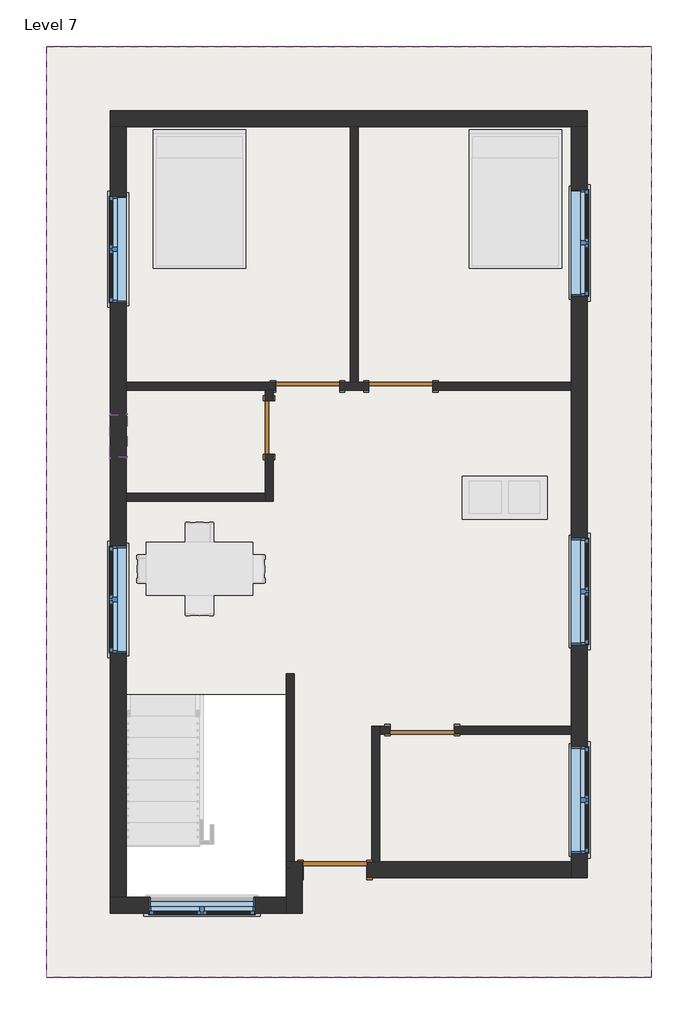
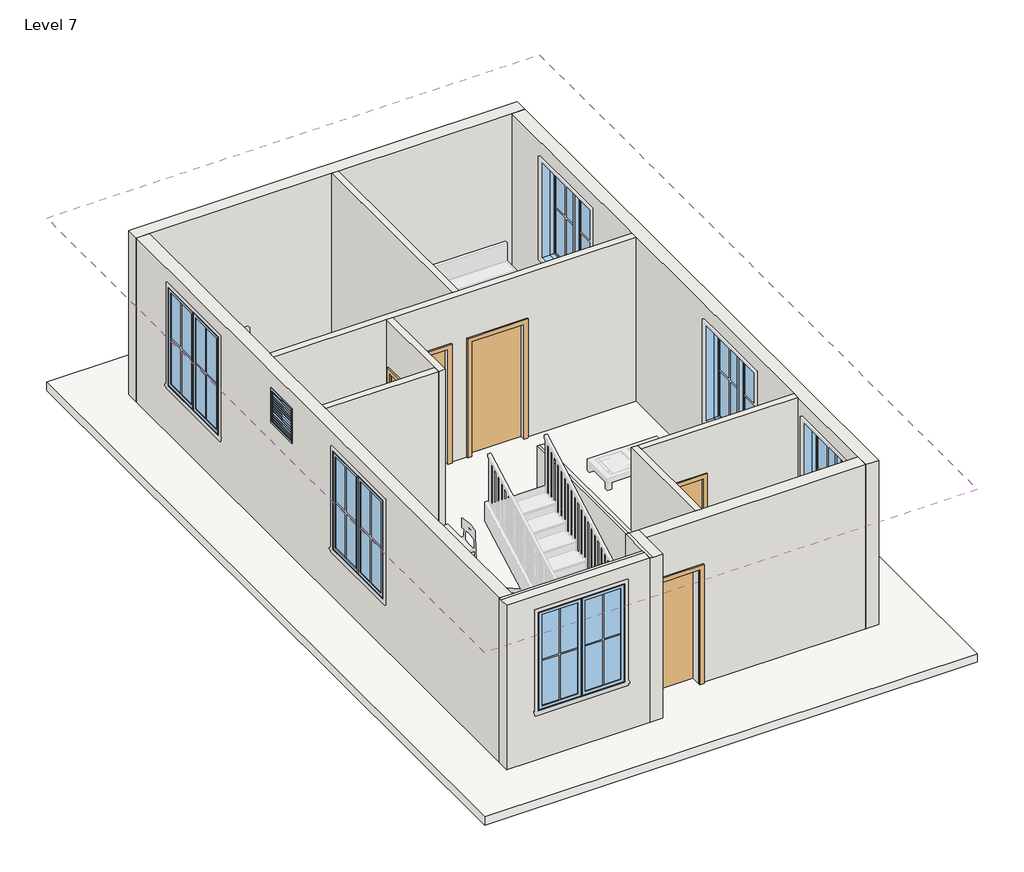
# One storey, part 1 of 3: 13 walls, 7 windows, 5 doors, 2 roofs.
"""IFC4 building model written with IfcOpenShell, lengths in millimetres."""

from ifc_helpers import new_model, si_unit, frame, origin, place, context, project, spatial, polyline, outline, extrude, faceted_brep, transform, mapped, element, save
from components import door_214872d5, single_flush_door_3_e5f9f3c4, single_flush_door_3_305aa2a5, single_flush_door_3_0ca8825f, window_casement_double_win_5_f93960c7, window_f2d8fef0

model = new_model("IFC4")

# Units and contexts
model_context = context("Model", 3, world=origin())
ifc_project = project(units=[si_unit("LENGTHUNIT", "METRE", prefix="MILLI")], contexts=[model_context])

# Site, building, storey
site = spatial("IfcSite", under=ifc_project)
building = spatial("IfcBuilding", under=site)
storey = spatial("IfcBuildingStorey", under=building, Name="Level 7", Elevation=19050.0)

# Doors
placement = place(None, origin())
door_shape = door_214872d5(model_context)
element("IfcDoor", 1, ObjectType="Single-Flush : DOOR 2'6\"", at=placement, inside=storey, context=model_context, shape_type="MappedRepresentation", body=[
    mapped(door_shape, transform((-2193.930864, 251.0919982, 19050.0), x_axis=(0.0, 1.0, 0.0), y_axis=(-1.0, 0.0, 0.0), z_axis=(0.0, 0.0, 1.0))),
])
single_flush_door_3_shape = single_flush_door_3_e5f9f3c4(model_context)
element("IfcDoor", 2, ObjectType="Single-Flush : DOOR 3'", at=placement, inside=storey, context=model_context, shape_type="MappedRepresentation", body=[
    mapped(single_flush_door_3_shape, transform((-1641.3962678, 841.6419982, 19050.0), x_axis=(1.0, 0.0, 0.0), y_axis=(0.0, 1.0, 0.0), z_axis=(0.0, 0.0, 1.0))),
])
element("IfcDoor", 3, ObjectType="Single-Flush : DOOR 3'", at=placement, inside=storey, context=model_context, shape_type="MappedRepresentation", body=[
    mapped(single_flush_door_3_shape, transform((-3.180864, -4073.2580018, 19050.0), x_axis=(-1.0, 0.0, 0.0), y_axis=(0.0, -1.0, 0.0), z_axis=(0.0, 0.0, 1.0))),
])
single_flush_door_3_2_shape = single_flush_door_3_305aa2a5(model_context)
element("IfcDoor", 4, ObjectType="Single-Flush : DOOR 3'", at=placement, inside=storey, context=model_context, shape_type="MappedRepresentation", body=[
    mapped(single_flush_door_3_2_shape, transform((-307.980864, 841.6419982, 19050.0), x_axis=(-1.0, 0.0, 0.0), y_axis=(0.0, -1.0, 0.0), z_axis=(0.0, 0.0, 1.0))),
])
single_flush_door_3_3_shape = single_flush_door_3_0ca8825f(model_context)
element("IfcDoor", 5, ObjectType="Single-Flush : DOOR 3'", at=placement, inside=storey, context=model_context, shape_type="MappedRepresentation", body=[
    mapped(single_flush_door_3_3_shape, transform((-1250.955864, -6073.5080018, 19050.0), x_axis=(1.0, 0.0, 0.0), y_axis=(0.0, 1.0, 0.0), z_axis=(0.0, 0.0, 1.0))),
])

# Roofs
element("IfcRoof", 6, ObjectType="ROOF 6\"", at=placement, inside=storey, context=model_context, shape_type="SweptSolid", body=[
    extrude(outline(polyline([(3273.419136, 5699.3919982), (3273.419136, -7610.2080018), (-5375.280864, -7610.2080018), (-5375.280864, 5699.3919982), (3273.419136, 5699.3919982)]), holes=[polyline([(-1895.480864, -3571.6080018), (-4232.280864, -3571.6080018), (-4232.280864, -6518.0080018), (-1895.480864, -6518.0080018), (-1895.480864, -3571.6080018)])]), frame((0.0, 0.0, 18897.6), z_axis=(0.0, 0.0, 1.0), x_axis=(1.0, 0.0, 0.0)), (0.0, 0.0, 1.0), 152.4),
])
element("IfcRoof", 7, ObjectType="ROOF 6\"", at=placement, inside=storey, context=model_context, shape_type="SweptSolid", body=[
    extrude(outline(polyline([(3273.419136, 5699.3919982), (3273.419136, -7610.2080018), (-5375.280864, -7610.2080018), (-5375.280864, 5699.3919982), (3273.419136, 5699.3919982)]), holes=[polyline([(-1895.480864, -3571.6080018), (-4232.280864, -3571.6080018), (-4232.280864, -6518.0080018), (-1895.480864, -6518.0080018), (-1895.480864, -3571.6080018)])]), frame((0.0, 0.0, 22098.0), z_axis=(0.0, 0.0, 1.0), x_axis=(1.0, 0.0, 0.0)), (0.0, 0.0, 1.0), 152.4),
])

# Walls
element("IfcWall", 8, ObjectType="WALL 4.5\"", at=placement, inside=storey, context=model_context, shape_type="SweptSolid", body=[
    extrude(outline(polyline([(-1031.880864, 898.7919982), (-1031.880864, 4556.3919982), (-917.580864, 4556.3919982), (-917.580864, 898.7919982), (-1031.880864, 898.7919982)])), frame((0.0, 0.0, 19050.0), z_axis=(0.0, 0.0, 1.0), x_axis=(1.0, 0.0, 0.0)), (0.0, 0.0, 1.0), 3048.0),
])
element("IfcWall", 9, ObjectType="WALL 4.5\"", at=placement, inside=storey, context=model_context, shape_type="Brep", body=[
    faceted_brep([(-765.180864, 898.7919982, 21183.6), (-765.180864, 898.7919982, 19050.0), (-917.580864, 898.7919982, 19050.0), (-1031.880864, 898.7919982, 19050.0), (-1184.1962678, 898.7919982, 19050.0), (-1184.1962678, 898.7919982, 21183.6), (-2098.5962678, 898.7919982, 21183.6), (-2098.5962678, 898.7919982, 19050.0), (-4232.280864, 898.7919982, 19050.0), (-4232.280864, 898.7919982, 22098.0), (-1031.880864, 898.7919982, 22098.0), (-917.580864, 898.7919982, 22098.0), (2130.419136, 898.7919982, 22098.0), (2130.419136, 898.7919982, 19050.0), (149.219136, 898.7919982, 19050.0), (149.219136, 898.7919982, 21183.6), (-1184.1962678, 784.4919982, 19050.0), (-765.180864, 784.4919982, 19050.0), (-765.180864, 784.4919982, 21183.6), (149.219136, 784.4919982, 21183.6), (149.219136, 784.4919982, 19050.0), (2130.419136, 784.4919982, 19050.0), (2130.419136, 784.4919982, 22098.0), (-2136.780864, 784.4919982, 22098.0), (-2251.080864, 784.4919982, 22098.0), (-4232.280864, 784.4919982, 22098.0), (-4232.280864, 784.4919982, 19050.0), (-2251.080864, 784.4919982, 19050.0), (-2136.780864, 784.4919982, 19050.0), (-2098.5962678, 784.4919982, 19050.0), (-2098.5962678, 784.4919982, 21183.6), (-1184.1962678, 784.4919982, 21183.6)], [[[0, 1, 2, 3, 4, 5, 6, 7, 8, 9, 10, 11, 12, 13, 14, 15]], [[16, 17, 18, 19, 20, 21, 22, 23, 24, 25, 26, 27, 28, 29, 30, 31]], [[29, 28, 27, 26, 8, 7]], [[14, 13, 21, 20]], [[4, 3, 2, 1, 17, 16]], [[13, 12, 22, 21]], [[9, 8, 26, 25]], [[5, 4, 16, 31]], [[6, 5, 31, 30]], [[7, 6, 30, 29]], [[18, 17, 1, 0]], [[19, 18, 0, 15]], [[20, 19, 15, 14]], [[12, 11, 10, 9, 25, 24, 23, 22]]]),
])
element("IfcWall", 10, ObjectType="WALL 4.5\"", at=placement, inside=storey, context=model_context, shape_type="Brep", body=[
    faceted_brep([(-2251.080864, 784.4919982, 19050.0), (-2251.080864, 632.0919982, 19050.0), (-2251.080864, 632.0919982, 21183.6), (-2251.080864, -129.9080018, 21183.6), (-2251.080864, -129.9080018, 19050.0), (-2251.080864, -688.7080018, 19050.0), (-2251.080864, -803.0080018, 19050.0), (-2251.080864, -803.0080018, 22098.0), (-2251.080864, -688.7080018, 22098.0), (-2251.080864, 784.4919982, 22098.0), (-2136.780864, 632.0919982, 21183.6), (-2136.780864, 632.0919982, 19050.0), (-2136.780864, 784.4919982, 19050.0), (-2136.780864, 784.4919982, 22098.0), (-2136.780864, -803.0080018, 22098.0), (-2136.780864, -803.0080018, 19050.0), (-2136.780864, -129.9080018, 19050.0), (-2136.780864, -129.9080018, 21183.6)], [[[0, 1, 2, 3, 4, 5, 6, 7, 8, 9]], [[10, 11, 12, 13, 14, 15, 16, 17]], [[16, 15, 6, 5, 4]], [[12, 11, 1, 0]], [[0, 9, 13, 12]], [[7, 6, 15, 14]], [[2, 1, 11, 10]], [[3, 2, 10, 17]], [[4, 3, 17, 16]], [[9, 8, 7, 14, 13]]]),
])
element("IfcWall", 11, ObjectType="WALL 4.5\"", at=placement, inside=storey, context=model_context, shape_type="SweptSolid", body=[
    extrude(outline(polyline([(-4232.280864, -688.7080018), (-2251.080864, -688.7080018), (-2251.080864, -803.0080018), (-4232.280864, -803.0080018), (-4232.280864, -688.7080018)])), frame((0.0, 0.0, 19050.0), z_axis=(0.0, 0.0, 1.0), x_axis=(1.0, 0.0, 0.0)), (0.0, 0.0, 1.0), 3048.0),
])
element("IfcWall", 12, ObjectType="WALL 4.5\"", at=placement, inside=storey, context=model_context, shape_type="Brep", body=[
    faceted_brep([(-1831.980864, -5959.2080018, 19050.0), (-1831.980864, -3266.8080018, 19050.0), (-1831.980864, -3266.8080018, 22098.0), (-1831.980864, -5959.2080018, 22098.0), (-1946.280864, -5959.2080018, 19050.0), (-1946.280864, -5959.2080018, 22098.0), (-1946.280864, -3266.8080018, 22098.0), (-1946.280864, -3266.8080018, 19050.0), (-1895.480864, -3266.8080018, 22098.0), (-1895.480864, -5959.2080018, 22098.0), (-1895.480864, -3571.6080018, 22098.0)], [[[0, 1, 2, 3]], [[4, 5, 6, 7]], [[1, 0, 4, 7]], [[2, 1, 7, 6, 8]], [[0, 3, 9, 5, 4]], [[3, 2, 8, 10, 9]], [[8, 6, 5, 9, 10]]]),
])
element("IfcWall", 13, ObjectType="WALL 4.5\"", at=placement, inside=storey, context=model_context, shape_type="Brep", body=[
    faceted_brep([(-612.780864, -5959.2080018, 19050.0), (-612.780864, -4130.4080018, 19050.0), (-612.780864, -4016.1080018, 19050.0), (-612.780864, -4016.1080018, 22098.0), (-612.780864, -4130.4080018, 22098.0), (-612.780864, -5959.2080018, 22098.0), (-727.080864, -5959.2080018, 19050.0), (-727.080864, -5959.2080018, 22098.0), (-727.080864, -4016.1080018, 22098.0), (-727.080864, -4016.1080018, 19050.0)], [[[0, 1, 2, 3, 4, 5]], [[6, 7, 8, 9]], [[2, 1, 0, 6, 9]], [[0, 5, 7, 6]], [[3, 2, 9, 8]], [[5, 4, 3, 8, 7]]]),
])
element("IfcWall", 14, ObjectType="WALL 4.5\"", at=placement, inside=storey, context=model_context, shape_type="SweptSolid", body=[
    extrude(outline(polyline([(19050.0, -612.780864), (19050.0, -460.380864), (21183.6, -460.380864), (21183.6, 454.019136), (19050.0, 454.019136), (19050.0, 2130.419136), (22098.0, 2130.419136), (22098.0, -612.780864), (19050.0, -612.780864)])), frame((0.0, -4130.4080018, 0.0), z_axis=(0.0, 1.0, 0.0), x_axis=(0.0, 0.0, 1.0)), (0.0, 0.0, 1.0), 114.3),
])
element("IfcWall", 15, ObjectType="WALL 9\"", at=placement, inside=storey, context=model_context, shape_type="Brep", body=[
    faceted_brep([(-4460.880864, 4556.3919982, 19050.0), (-4232.280864, 4556.3919982, 19050.0), (-1031.880864, 4556.3919982, 19050.0), (-917.580864, 4556.3919982, 19050.0), (2130.419136, 4556.3919982, 19050.0), (2359.019136, 4556.3919982, 19050.0), (2359.019136, 4556.3919982, 22098.0), (2130.419136, 4556.3919982, 22098.0), (-917.580864, 4556.3919982, 22098.0), (-1031.880864, 4556.3919982, 22098.0), (-4232.280864, 4556.3919982, 22098.0), (-4460.880864, 4556.3919982, 22098.0), (-4460.880864, 4784.9919982, 19050.0), (-4460.880864, 4784.9919982, 22098.0), (2359.019136, 4784.9919982, 22098.0), (2359.019136, 4784.9919982, 19050.0)], [[[0, 1, 2, 3, 4, 5, 6, 7, 8, 9, 10, 11]], [[12, 13, 14, 15]], [[5, 4, 3, 2, 1, 0, 12, 15]], [[6, 5, 15, 14]], [[0, 11, 13, 12]], [[11, 10, 9, 8, 7, 6, 14, 13]]]),
])
element("IfcWall", 16, ObjectType="WALL 9\"", at=placement, inside=storey, context=model_context, shape_type="Brep", body=[
    faceted_brep([(2130.419136, 4556.3919982, 19050.0), (2130.419136, 898.7919982, 19050.0), (2130.419136, 784.4919982, 19050.0), (2130.419136, -4016.1080018, 19050.0), (2130.419136, -4130.4080018, 19050.0), (2130.419136, -5959.2080018, 19050.0), (2130.419136, -6187.8080018, 19050.0), (2130.419136, -6187.8080018, 22098.0), (2130.419136, -5959.2080018, 22098.0), (2130.419136, -4130.4080018, 22098.0), (2130.419136, -4016.1080018, 22098.0), (2130.419136, 784.4919982, 22098.0), (2130.419136, 898.7919982, 22098.0), (2130.419136, 4556.3919982, 22098.0), (2130.419136, -5835.3830018, 21793.2), (2130.419136, -5835.3830018, 19964.4), (2130.419136, -4311.3830018, 19964.4), (2130.419136, -4311.3830018, 21793.2), (2130.419136, -2854.0580018, 21793.2), (2130.419136, -2854.0580018, 19964.4), (2130.419136, -1330.0580018, 19964.4), (2130.419136, -1330.0580018, 21793.2), (2130.419136, 2130.6919982, 21793.2), (2130.419136, 2130.6919982, 19964.4), (2130.419136, 3654.6919982, 19964.4), (2130.419136, 3654.6919982, 21793.2), (2359.019136, 4556.3919982, 19050.0), (2359.019136, 4556.3919982, 22098.0), (2359.019136, -6187.8080018, 22098.0), (2359.019136, -6187.8080018, 19050.0), (2359.019136, -5835.3830018, 21793.2), (2359.019136, -4311.3830018, 21793.2), (2359.019136, -4311.3830018, 19964.4), (2359.019136, -5835.3830018, 19964.4), (2359.019136, -2854.0580018, 21793.2), (2359.019136, -1330.0580018, 21793.2), (2359.019136, -1330.0580018, 19964.4), (2359.019136, -2854.0580018, 19964.4), (2359.019136, 2130.6919982, 21793.2), (2359.019136, 3654.6919982, 21793.2), (2359.019136, 3654.6919982, 19964.4), (2359.019136, 2130.6919982, 19964.4)], [[[0, 1, 2, 3, 4, 5, 6, 7, 8, 9, 10, 11, 12, 13], [14, 15, 16, 17], [18, 19, 20, 21], [22, 23, 24, 25]], [[26, 27, 28, 29], [30, 31, 32, 33], [34, 35, 36, 37], [38, 39, 40, 41]], [[6, 5, 4, 3, 2, 1, 0, 26, 29]], [[0, 13, 27, 26]], [[7, 6, 29, 28]], [[15, 14, 30, 33]], [[16, 15, 33, 32]], [[17, 16, 32, 31]], [[14, 17, 31, 30]], [[19, 18, 34, 37]], [[20, 19, 37, 36]], [[21, 20, 36, 35]], [[18, 21, 35, 34]], [[23, 22, 38, 41]], [[24, 23, 41, 40]], [[25, 24, 40, 39]], [[22, 25, 39, 38]], [[13, 12, 11, 10, 9, 8, 7, 28, 27]]]),
])
element("IfcWall", 17, ObjectType="WALL 9\"", at=placement, inside=storey, context=model_context, shape_type="Brep", body=[
    faceted_brep([(2130.419136, -5959.2080018, 19050.0), (-612.780864, -5959.2080018, 19050.0), (-727.080864, -5959.2080018, 19050.0), (-793.755864, -5959.2080018, 19050.0), (-793.755864, -5959.2080018, 21183.6), (-1708.155864, -5959.2080018, 21183.6), (-1708.155864, -5959.2080018, 19050.0), (-1717.680864, -5959.2080018, 19050.0), (-1717.680864, -5959.2080018, 22098.0), (-727.080864, -5959.2080018, 22098.0), (-612.780864, -5959.2080018, 22098.0), (2130.419136, -5959.2080018, 22098.0), (-793.755864, -6187.8080018, 21183.6), (-793.755864, -6187.8080018, 19050.0), (2130.419136, -6187.8080018, 19050.0), (2130.419136, -6187.8080018, 22098.0), (-1717.680864, -6187.8080018, 22098.0), (-1717.680864, -6187.8080018, 19050.0), (-1708.155864, -6187.8080018, 19050.0), (-1708.155864, -6187.8080018, 21183.6)], [[[0, 1, 2, 3, 4, 5, 6, 7, 8, 9, 10, 11]], [[12, 13, 14, 15, 16, 17, 18, 19]], [[18, 17, 7, 6]], [[14, 13, 3, 2, 1, 0]], [[0, 11, 15, 14]], [[8, 7, 17, 16]], [[4, 3, 13, 12]], [[5, 4, 12, 19]], [[6, 5, 19, 18]], [[11, 10, 9, 8, 16, 15]]]),
])
element("IfcWall", 18, ObjectType="WALL 9\"", at=placement, inside=storey, context=model_context, shape_type="Brep", body=[
    faceted_brep([(-1946.280864, -5959.2080018, 19050.0), (-1946.280864, -6467.2080018, 19050.0), (-1946.280864, -6695.8080018, 19050.0), (-1946.280864, -6695.8080018, 22098.0), (-1946.280864, -6467.2080018, 22098.0), (-1946.280864, -5959.2080018, 22098.0), (-1717.680864, -5959.2080018, 19050.0), (-1717.680864, -5959.2080018, 22098.0), (-1717.680864, -6187.8080018, 22098.0), (-1717.680864, -6695.8080018, 22098.0), (-1717.680864, -6695.8080018, 19050.0), (-1717.680864, -6187.8080018, 19050.0), (-1831.980864, -5959.2080018, 19050.0), (-1895.480864, -5959.2080018, 22098.0), (-1831.980864, -5959.2080018, 22098.0), (-1895.480864, -6695.8080018, 22098.0), (-1895.480864, -6518.0080018, 22098.0)], [[[0, 1, 2, 3, 4, 5]], [[6, 7, 8, 9, 10, 11]], [[2, 1, 0, 12, 6, 11, 10]], [[0, 5, 13, 14, 7, 6, 12]], [[3, 2, 10, 9, 15]], [[5, 4, 3, 15, 16, 13]], [[15, 9, 8, 7, 14, 13, 16]]]),
])
element("IfcWall", 19, ObjectType="WALL 9\"", at=placement, inside=storey, context=model_context, shape_type="Brep", body=[
    faceted_brep([(-1946.280864, -6467.2080018, 19050.0), (-4232.280864, -6467.2080018, 19050.0), (-4460.880864, -6467.2080018, 19050.0), (-4460.880864, -6467.2080018, 22098.0), (-4232.280864, -6467.2080018, 22098.0), (-1946.280864, -6467.2080018, 22098.0), (-3914.780864, -6467.2080018, 21793.2), (-3914.780864, -6467.2080018, 19964.4), (-2390.780864, -6467.2080018, 19964.4), (-2390.780864, -6467.2080018, 21793.2), (-1946.280864, -6695.8080018, 19050.0), (-1946.280864, -6695.8080018, 22098.0), (-4460.880864, -6695.8080018, 22098.0), (-4460.880864, -6695.8080018, 19050.0), (-3914.780864, -6695.8080018, 21793.2), (-2390.780864, -6695.8080018, 21793.2), (-2390.780864, -6695.8080018, 19964.4), (-3914.780864, -6695.8080018, 19964.4), (-1946.280864, -6518.0080018, 22098.0), (-4460.880864, -6518.0080018, 22098.0), (-4232.280864, -6518.0080018, 22098.0)], [[[0, 1, 2, 3, 4, 5], [6, 7, 8, 9]], [[10, 11, 12, 13], [14, 15, 16, 17]], [[2, 1, 0, 10, 13]], [[0, 5, 18, 11, 10]], [[3, 2, 13, 12, 19]], [[7, 6, 14, 17]], [[8, 7, 17, 16]], [[9, 8, 16, 15]], [[6, 9, 15, 14]], [[5, 4, 3, 19, 20, 18]], [[19, 12, 11, 18, 20]]]),
])
element("IfcWall", 20, ObjectType="WALL 9\"", at=placement, inside=storey, context=model_context, shape_type="Brep", body=[
    faceted_brep([(-4232.280864, -6467.2080018, 19050.0), (-4232.280864, -803.0080018, 19050.0), (-4232.280864, -688.7080018, 19050.0), (-4232.280864, 784.4919982, 19050.0), (-4232.280864, 898.7919982, 19050.0), (-4232.280864, 4556.3919982, 19050.0), (-4232.280864, 4556.3919982, 22098.0), (-4232.280864, 898.7919982, 22098.0), (-4232.280864, 784.4919982, 22098.0), (-4232.280864, -688.7080018, 22098.0), (-4232.280864, -803.0080018, 22098.0), (-4232.280864, -3571.6080018, 22098.0), (-4232.280864, -6467.2080018, 22098.0), (-4232.280864, -1445.1400081, 21793.2), (-4232.280864, -1445.1400081, 19964.4), (-4232.280864, -2969.1400081, 19964.4), (-4232.280864, -2969.1400081, 21793.2), (-4232.280864, 3562.6287133, 21793.2), (-4232.280864, 3562.6287133, 19964.4), (-4232.280864, 2038.6287133, 19964.4), (-4232.280864, 2038.6287133, 21793.2), (-4232.280864, -174.3580018, 21793.2), (-4232.280864, 435.2419982, 21793.2), (-4232.280864, 435.2419982, 21183.6), (-4232.280864, -174.3580018, 21183.6), (-4460.880864, -6467.2080018, 19050.0), (-4460.880864, -6467.2080018, 22098.0), (-4460.880864, 4556.3919982, 22098.0), (-4460.880864, 4556.3919982, 19050.0), (-4460.880864, -1445.1400081, 21793.2), (-4460.880864, -2969.1400081, 21793.2), (-4460.880864, -2969.1400081, 19964.4), (-4460.880864, -1445.1400081, 19964.4), (-4460.880864, 3562.6287133, 21793.2), (-4460.880864, 2038.6287133, 21793.2), (-4460.880864, 2038.6287133, 19964.4), (-4460.880864, 3562.6287133, 19964.4), (-4460.880864, -174.3580018, 21793.2), (-4460.880864, -174.3580018, 21183.6), (-4460.880864, 435.2419982, 21183.6), (-4460.880864, 435.2419982, 21793.2)], [[[0, 1, 2, 3, 4, 5, 6, 7, 8, 9, 10, 11, 12], [13, 14, 15, 16], [17, 18, 19, 20], [21, 22, 23, 24]], [[25, 26, 27, 28], [29, 30, 31, 32], [33, 34, 35, 36], [37, 38, 39, 40]], [[5, 4, 3, 2, 1, 0, 25, 28]], [[6, 5, 28, 27]], [[0, 12, 26, 25]], [[14, 13, 29, 32]], [[15, 14, 32, 31]], [[16, 15, 31, 30]], [[13, 16, 30, 29]], [[18, 17, 33, 36]], [[19, 18, 36, 35]], [[20, 19, 35, 34]], [[17, 20, 34, 33]], [[38, 37, 21, 24]], [[39, 38, 24, 23]], [[40, 39, 23, 22]], [[37, 40, 22, 21]], [[12, 11, 10, 9, 8, 7, 6, 27, 26]]]),
])

# Windows
window_casement_double_win_5_shape = window_casement_double_win_5_f93960c7(model_context)
element("IfcWindow", 21, ObjectType="Window-Casement-Double : WIN 5'", at=placement, inside=storey, context=model_context, shape_type="MappedRepresentation", body=[
    mapped(window_casement_double_win_5_shape, transform((-3152.780864, -6581.5080018, 19050.0), x_axis=(-1.0, 0.0, 0.0), y_axis=(0.0, -1.0, 0.0), z_axis=(0.0, 0.0, 1.0))),
])
element("IfcWindow", 22, ObjectType="Window-Casement-Double : WIN 5'", at=placement, inside=storey, context=model_context, shape_type="MappedRepresentation", body=[
    mapped(window_casement_double_win_5_shape, transform((2244.719136, -5073.3830018, 19050.0), x_axis=(0.0, -1.0, 0.0), y_axis=(1.0, 0.0, 0.0), z_axis=(0.0, 0.0, 1.0))),
])
element("IfcWindow", 23, ObjectType="Window-Casement-Double : WIN 5'", at=placement, inside=storey, context=model_context, shape_type="MappedRepresentation", body=[
    mapped(window_casement_double_win_5_shape, transform((2244.719136, -2092.0580018, 19050.0), x_axis=(0.0, -1.0, 0.0), y_axis=(1.0, 0.0, 0.0), z_axis=(0.0, 0.0, 1.0))),
])
element("IfcWindow", 24, ObjectType="Window-Casement-Double : WIN 5'", at=placement, inside=storey, context=model_context, shape_type="MappedRepresentation", body=[
    mapped(window_casement_double_win_5_shape, transform((-4346.580864, -2207.1400081, 19050.0), x_axis=(0.0, 1.0, 0.0), y_axis=(-1.0, 0.0, 0.0), z_axis=(0.0, 0.0, 1.0))),
])
element("IfcWindow", 25, ObjectType="Window-Casement-Double : WIN 5'", at=placement, inside=storey, context=model_context, shape_type="MappedRepresentation", body=[
    mapped(window_casement_double_win_5_shape, transform((2244.719136, 2892.6919982, 19050.0), x_axis=(0.0, -1.0, 0.0), y_axis=(1.0, 0.0, 0.0), z_axis=(0.0, 0.0, 1.0))),
])
element("IfcWindow", 26, ObjectType="Window-Casement-Double : WIN 5'", at=placement, inside=storey, context=model_context, shape_type="MappedRepresentation", body=[
    mapped(window_casement_double_win_5_shape, transform((-4346.580864, 2800.6287133, 19050.0), x_axis=(0.0, 1.0, 0.0), y_axis=(-1.0, 0.0, 0.0), z_axis=(0.0, 0.0, 1.0))),
])
window_shape = window_f2d8fef0(model_context)
element("IfcWindow", 27, ObjectType="Window-Louvers : 24\" x 24\"", at=placement, inside=storey, context=model_context, shape_type="MappedRepresentation", body=[
    mapped(window_shape, transform((-4352.930864, 130.4419982, 20269.2), x_axis=(0.0, 1.0, 0.0), y_axis=(-1.0, 0.0, 0.0), z_axis=(0.0, 0.0, 1.0))),
])

save(model, "model.ifc")

# Revit data of these elements
# Type "Single-Flush : DOOR 2'6\""
#   Type Mark = "9"
#   Construction Type Id = "MDOOR"
#   Assembly Code = "C1020"
#   Analytic Construction = "Metal"
#   Thickness = 0' - 2"
#   Heat Transfer Coefficient (U) = 0.651978 BTU/(h·ft²·°F)
#   Height = 7' - 0"
#   Trim Projection Ext = 0' - 1"
#   Trim Projection Int = 0' - 1"
#   Trim Width = 0' - 3"
#   Width = 2' - 6"
#   Define Thermal Properties by = 1
#   Door Material = Door - Panel
#   Frame Material = Door - Frame
#   Visual Light Transmittance = 0
#   Solar Heat Gain Coefficient = 0
#   Function = (empty or 0)
#   Wall Closure = (empty or 0)
# Type "Single-Flush : DOOR 3'"
#   Type Mark = "8"
#   Construction Type Id = "MDOOR"
#   Assembly Code = "C1020"
#   Analytic Construction = "Metal"
#   Thickness = 0' - 2"
#   Heat Transfer Coefficient (U) = 0.651978 BTU/(h·ft²·°F)
#   Height = 7' - 0"
#   Trim Projection Ext = 0' - 1"
#   Trim Projection Int = 0' - 1"
#   Trim Width = 0' - 3"
#   Width = 3' - 0"
#   Define Thermal Properties by = 1
#   Door Material = Door - Panel
#   Frame Material = Door - Frame
#   Visual Light Transmittance = 0
#   Solar Heat Gain Coefficient = 0
#   Function = (empty or 0)
#   Wall Closure = (empty or 0)
# Type "ROOF 6\""
#   Assembly Code = "B1020"
#   Layers, outside or top first: 0' - 6" no material (function 1)
# Type "WALL 4.5\""
#   Assembly Code = "B2010"
#   Layers, outside or top first: 0' - 4 1/2" no material (function 1)
# Type "WALL 9\""
#   Assembly Code = "B2010"
#   Layers, outside or top first: 0' - 9" no material (function 1)
# Type "Window-Casement-Double : WIN 5'"
#   Type Mark = "18"
#   Fire Rating = "0.5h"
#   Assembly Code = "B2020100"
#   Analytic Construction = "Double glazing - domestic"
#   Frame Extension [instance default] = 0' - 0 1/4"
#   Window Inset [instance default] = 0' - 0"
#   Wall Thickness [instance default] = 0' - 6"
#   Interior Wall Closure [instance default] = 0' - 2 1/4"
#   Half Width = 2' - 6"
#   Visual Light Transmittance = 0.81
#   Thermal Resistance (R) = 1.8146 (h·ft²·°F)/BTU
#   Solar Heat Gain Coefficient = 0.76
#   Rough Width = 5' - 0 1/2"
#   Rough Height = 6' - 0 1/2"
#   Height = 6' - 0"
#   Heat Transfer Coefficient (U) = 0.5511 BTU/(h·ft²·°F)
#   Exterior Wall Closure [instance default] = 0' - 1 1/4"
#   Extension Jamb [instance default] = 0' - 2 1/4"
#   Default Sill Height = 3' - 0"
#   Width = 5' - 0"
#   Muntin Visibility = yes
#   Interior Trim Visibility [instance default] = yes
#   Exterior Trim Visibility [instance default] = yes
#   Extension Jamb Visibility [instance default] = yes
#   Interior Trim Material = Wood - Stained
#   Muntin Pattern = Muntin Pattern_2x2 : Muntin Pattern_2x2
#   Interior Trim = Trim-Window-Interior-Flat : Picture Frame
#   Interior Frame Material = Wood - Stained
#   Glass Panel Material = Glass
#   Exterior Trim Material = Clad - White
#   Exterior Trim = Trim-Window-Exterior-Flat : with Sill
#   Exterior Frame Material = Clad - White
#   Wall Closure = (empty or 0)
# Type "Window-Louvers : 24\" x 24\""
#   Type Mark = "19"
#   Construction Type Id = "GSP4R"
#   Assembly Code = "B20"
#   Analytic Construction = "1/8 in Pilkington single glazing"
#   Visual Light Transmittance = 0.9
#   Thermal Resistance (R) = 1.53941 (h·ft²·°F)/BTU
#   Solar Heat Gain Coefficient = 0.78
#   Max Height = 1' - 11.74264"
#   Height = 2' - 0"
#   Heat Transfer Coefficient (U) = 0.6496 BTU/(h·ft²·°F)
#   Blade Width [instance default] = 1' - 10 1/2"
#   Blade Vertical Thickness = 0' - 0.35355"
#   Blade Thickness = 0' - 0 1/4"
#   Blade Spacing = 0' - 1 1/2"
#   Blade Height = 0' - 1.85355"
#   Blade Depth = 0' - 3"
#   Blade Angle = 45.00°
#   Default Sill Height = 3' - 0"
#   Trim Projection_Exterior = 0' - 0 1/2"
#   Trim Projection_Interior = 0' - 0 1/2"
#   Trim Width_Exterior = 0' - 1 1/2"
#   Trim Width_Interior = 0' - 1 1/2"
#   Width = 2' - 0"
#   Max Blade Count = 12
#   Define Thermal Properties by = 1
#   Blade Count = 12
#   Frame Material = Birch
#   Louver Material = Birch
#   Trim Exterior Material = Birch
#   Trim Interior Material = Birch
#   Wall Closure = (empty or 0)
# Element 1 (IfcDoor, "Single-Flush : DOOR 2'6\"")
#   Phase Created = New Construction
#   Materials on its faces: "Door - Frame", "Door - Panel"
# Elements 2, 3, 4, 5 (IfcDoor, "Single-Flush : DOOR 3'")
#   Phase Created = New Construction
#   Materials on its faces: "Door - Frame", "Door - Panel"
# Element 6 (IfcRoof, "ROOF 6\"")
#   built-in parameter 1001705 = 62.5 (stored number, unit not read)
#   built-in parameter 1001701 = -0.5 (stored number, unit not read)
#   built-in parameter 1001710 = 33615
#   Phase Created = New Construction
#   Materials on its faces: "Copper", "Wood - Stained"
# Element 7 (IfcRoof, "ROOF 6\"")
#   built-in parameter 1001705 = 73 (stored number, unit not read)
#   built-in parameter 1001701 = 10 (stored number, unit not read)
#   built-in parameter 1001710 = 33615
#   Phase Created = New Construction
#   Materials on its faces: "Copper", "Wood - Stained"
# Elements 8, 9, 10, 11, 13, 14 (IfcWall, "WALL 4.5\"")
#   Top Offset = 0' - 0"
#   Base Offset = 0' - 0"
#   Unconnected Height = 10' - 0"
#   wall height = 10' - 0"
#   Phase Created = New Construction
#   Base Constraint = Level 7
#   Materials on its faces: "Default Wall"
# Element 12 (IfcWall, "WALL 4.5\"")
#   Top Offset = 0' - 0"
#   Base Offset = 0' - 0"
#   Unconnected Height = 10' - 0"
#   wall height = 10' - 0"
#   Phase Created = New Construction
#   Base Constraint = Level 7
#   Materials on its faces: "Default Wall", "Copper"
# Elements 15, 16, 17 (IfcWall, "WALL 9\"")
#   Top Offset = 0' - 0"
#   Base Offset = 0' - 0"
#   Unconnected Height = 10' - 0"
#   wall height = 10' - 0"
#   Phase Created = New Construction
#   Base Constraint = Level 7
#   Materials on its faces: "Default Wall"
# Elements 18, 19, 20 (IfcWall, "WALL 9\"")
#   Top Offset = 0' - 0"
#   Base Offset = 0' - 0"
#   Unconnected Height = 10' - 0"
#   wall height = 10' - 0"
#   Phase Created = New Construction
#   Base Constraint = Level 7
#   Materials on its faces: "Default Wall", "Copper"
# Element 21 (IfcWindow, "Window-Casement-Double : WIN 5'")
#   Mark = "43"
#   Window Inset = 0' - 0"
#   Interior Wall Closure = 0' - 2 1/4"
#   Frame Extension = 0' - 0 1/4"
#   Exterior Wall Closure = 0' - 1 1/4"
#   Interior Trim Visibility = yes
#   Exterior Trim Visibility = yes
#   Phase Created = New Construction
#   Materials on its faces: "Wood - Stained", "Glass", "Clad - White"
# Element 22 (IfcWindow, "Window-Casement-Double : WIN 5'")
#   Mark = "44"
#   Window Inset = 0' - 0"
#   Interior Wall Closure = 0' - 2 1/4"
#   Frame Extension = 0' - 0 1/4"
#   Exterior Wall Closure = 0' - 1 1/4"
#   Interior Trim Visibility = yes
#   Exterior Trim Visibility = yes
#   Phase Created = New Construction
#   Materials on its faces: "Wood - Stained", "Glass", "Clad - White"
# Element 23 (IfcWindow, "Window-Casement-Double : WIN 5'")
#   Mark = "45"
#   Window Inset = 0' - 0"
#   Interior Wall Closure = 0' - 2 1/4"
#   Frame Extension = 0' - 0 1/4"
#   Exterior Wall Closure = 0' - 1 1/4"
#   Interior Trim Visibility = yes
#   Exterior Trim Visibility = yes
#   Phase Created = New Construction
#   Materials on its faces: "Wood - Stained", "Glass", "Clad - White"
# Element 24 (IfcWindow, "Window-Casement-Double : WIN 5'")
#   Mark = "46"
#   Window Inset = 0' - 0"
#   Interior Wall Closure = 0' - 2 1/4"
#   Frame Extension = 0' - 0 1/4"
#   Exterior Wall Closure = 0' - 1 1/4"
#   Interior Trim Visibility = yes
#   Exterior Trim Visibility = yes
#   Phase Created = New Construction
#   Materials on its faces: "Wood - Stained", "Glass", "Clad - White"
# Element 25 (IfcWindow, "Window-Casement-Double : WIN 5'")
#   Mark = "47"
#   Window Inset = 0' - 0"
#   Interior Wall Closure = 0' - 2 1/4"
#   Frame Extension = 0' - 0 1/4"
#   Exterior Wall Closure = 0' - 1 1/4"
#   Interior Trim Visibility = yes
#   Exterior Trim Visibility = yes
#   Phase Created = New Construction
#   Materials on its faces: "Wood - Stained", "Glass", "Clad - White"
# Element 26 (IfcWindow, "Window-Casement-Double : WIN 5'")
#   Mark = "48"
#   Window Inset = 0' - 0"
#   Interior Wall Closure = 0' - 2 1/4"
#   Frame Extension = 0' - 0 1/4"
#   Exterior Wall Closure = 0' - 1 1/4"
#   Interior Trim Visibility = yes
#   Exterior Trim Visibility = yes
#   Phase Created = New Construction
#   Materials on its faces: "Wood - Stained", "Glass", "Clad - White"
# Element 27 (IfcWindow, "Window-Louvers : 24\" x 24\"")
#   Mark = "49"
#   Blade Width = 1' - 10 1/2"
#   Phase Created = New Construction
#   Materials on its faces: "Birch"
# Materials
#   "Door - Panel": class "Wood", colour RGB 210 159 95, transparency 0, Cost = 0
#   "Door - Frame": colour RGB 118 70 51, transparency 0, Cost = 0
#   "Wood - Stained": class "Wood", colour RGB 224 178 126, transparency 0, Cost = 0
#   "Glass": class "Glass", colour RGB 0 128 192, transparency 0.75, Description = "Soda Lime Glass", Cost = 0
#   "Clad - White": class "Wood", colour RGB 242 242 238, transparency 0, Cost = 0
#   "Birch": class "Wood", colour RGB 224 178 126, transparency 0, Description = "Betula Alleghaniensis", Cost = 0
#   "Copper": class "Metal", colour RGB 0 0 0, transparency 0, Description = "Copper, matte finish", Cost = 0
#   "Default Wall": colour RGB 128 128 128, transparency 0, Cost = 0
